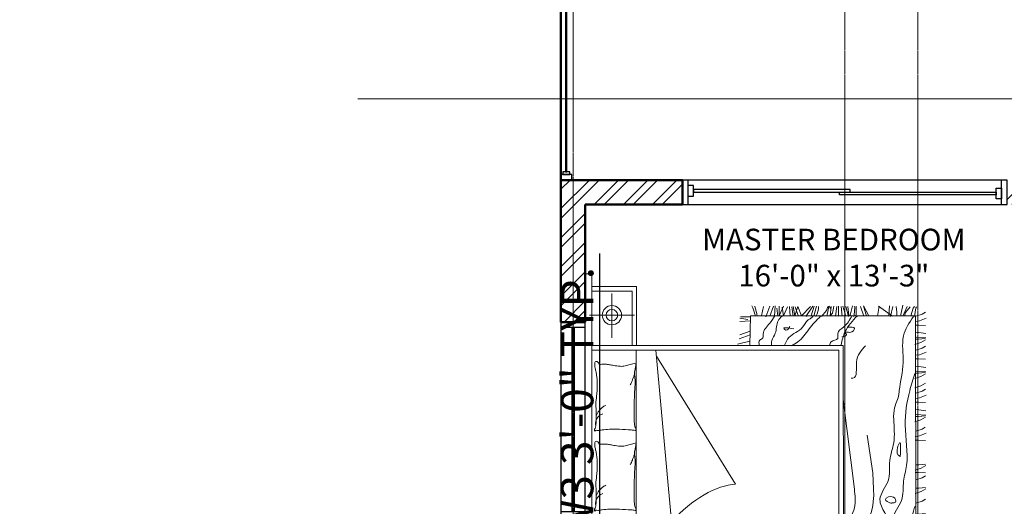
# Model space of a CAD drawing. Units: inches. Extents: x 261 to 2725, y 291 to 1454.
# Tile 22 of 35: x 1043 to 1407, y 853 to 1033. Entities that reach past the tile are written whole.
import ezdxf

# ---------------------------------------------------------------- set-up
doc = ezdxf.new("R2010")
doc.units = ezdxf.units.IN
doc.linetypes.add('CENTER', pattern=[2, 1.25, -0.25, 0.25, -0.25])
for name, color, linetype, lineweight in [('A-ANNO-DIMS', 136, 'Continuous', 18), ('A-AREA-IDEN', 18, 'Continuous', 18), ('A-DOOR', 160, 'Continuous', 25), ('A-FLOR-HRAL', 132, 'Continuous', 25), ('A-FURN', 30, 'Continuous', 18), ('A-GLAZ', 150, 'Continuous', 25), ('A-GRID', 251, 'CENTER', 13), ('A-WALL', 222, 'Continuous', 50), ('A-WALL-PATT', 243, 'Continuous', 13)]:
    doc.layers.add(name, color=color, linetype=linetype, lineweight=lineweight)
doc.styles.get("Standard").update_dxf_attribs({"font": 'arial.ttf'})
doc.dimstyles.new('ISO-25', dxfattribs={"dimtxt": 12, "dimasz": 6, "dimexe": 1.25, "dimexo": 0.625, "dimtad": 1, "dimdec": 0, "dimlunit": 3, "dimtxsty": 'Standard', "dimblk": 'ARCHTICK', "dimcen": 2.5, "dimadec": 0, "dimazin": 0, "dimtfac": 1, "dimtdec": 0, "dimtmove": 0, "dimatfit": 3, "dimfxl": 1, "dimfxlon": 1, "dimarcsym": 0})

# ---------------------------------------------------------------- blocks, each defined once
blk = doc.blocks.new('A$C2B723114')
for p, q in [((0, 2.9047), (2.8274, 2.9047)), ((0, 2.8487), (0, 2.9047)), ((0.4243, 2.8697), (0.4243, 2.4855)), ((2.4742, 2.8697), (2.4742, 2.4855)), ((2.8274, 2.9047), (2.8274, 2.8487)), ((2.8274, 2.8487), (0, 2.8487)), ((0.1012, 2.4649), (0.1012, 2.849)), ((0.1396, 2.5033), (0.1396, 2.849)), ((0.6794, 0.7051), (0.6794, 2.8509)), ((0.7187, 0.7435), (0.7187, 2.8509)), ((2.1776, 2.8509), (2.1776, 0.7454)), ((2.216, 2.8509), (2.216, 0.707)), ((2.6798, 2.5052), (2.6798, 2.8509)), ((2.7182, 2.4668), (2.7182, 2.8509)), ((0.6087, 2.6776), (0.295, 2.6776)), ((2.6586, 2.6776), (2.2821, 2.6776)), ((1.3789, 2.4999), (1.3598, 2.5761)), ((2.0593, 2.4999), (2.0402, 2.5761)), ((0.6794, 2.4649), (0.1012, 2.4649)), ((0.6766, 2.5033), (0.1396, 2.5033)), ((0.7191, 2.47), (2.1778, 2.4719)), ((1.3858, 2.4723), (1.3789, 2.4999)), ((2.0662, 2.4723), (2.0593, 2.4999)), ((2.2188, 2.5052), (2.6798, 2.5052)), ((2.2188, 2.4668), (2.7182, 2.4668)), ((2.1771, 2.3036), (0.718, 2.1685)), ((1.0365, 1.6233), (2.1246, 2.2989)), ((2.2287, 1.6076), (2.2523, 1.5035)), ((0.5047, 1.5819), (0.5353, 1.4945)), ((0.6174, 1.5819), (0.6232, 1.4916)), ((0.6467, 1.5819), (0.6369, 1.5137)), ((0.6571, 1.4945), (0.6571, 1.5765)), ((2.2726, 1.593), (2.3061, 1.5007)), ((2.3067, 1.5881), (2.3373, 1.5007)), ((2.4194, 1.5881), (2.4251, 1.4979)), ((2.4487, 1.5881), (2.4389, 1.5199)), ((2.4591, 1.5007), (2.4591, 1.5828)), ((0.4269, 0.0884), (0.4269, 1.4945)), ((0.4269, 1.4945), (0.6794, 1.4945)), ((2.4685, 1.4964), (2.216, 1.5022)), ((2.4685, 1.4964), (2.4685, 0.0903)), ((0.3172, 1.3923), (0.4213, 1.3687)), ((0.3318, 1.3485), (0.4241, 1.3149)), ((2.4596, 1.3659), (2.552, 1.3324)), ((2.4685, 1.4044), (2.5491, 1.3861)), ((0.3367, 1.3143), (0.4241, 1.2838)), ((2.4645, 1.3318), (2.552, 1.3012)), ((2.4645, 1.2928), (2.5548, 1.2871)), ((2.4645, 1.2635), (2.5328, 1.2733)), ((0.3367, 1.2016), (0.427, 1.1959)), ((0.3367, 1.1724), (0.405, 1.1821)), ((2.4699, 1.2531), (2.552, 1.2163)), ((2.552, 1.2531), (2.4699, 1.2531)), ((2.5435, 1.2276), (2.4699, 1.2163)), ((2.4699, 1.2163), (2.5463, 1.1823)), ((0.4241, 1.162), (0.3421, 1.162)), ((0.3421, 1.162), (0.4241, 1.1252)), ((2.5491, 1.1654), (2.467, 1.1597)), ((2.5463, 1.1455), (2.467, 1.1342)), ((2.5491, 1.1342), (2.4699, 1.1201)), ((2.4699, 1.1201), (2.5491, 1.0946)), ((2.5491, 1.0946), (2.4699, 1.0635)), ((2.5463, 1.1172), (2.4727, 1.0918)), ((0.4157, 1.0206), (0.3421, 1.0093)), ((0.3421, 1.0093), (0.4185, 0.9754)), ((2.4642, 1.0267), (2.552, 0.9644)), ((2.4699, 1.0635), (2.5491, 0.9842)), ((0.4213, 0.9584), (0.3392, 0.9527)), ((0.4185, 0.9386), (0.3392, 0.9272)), ((0.4213, 0.9272), (0.3421, 0.9131)), ((2.4642, 0.9389), (2.4869, 0.9276)), ((2.467, 0.9559), (2.552, 0.9333)), ((2.4699, 0.9785), (2.552, 0.9531)), ((2.4869, 0.9276), (2.5265, 0.9163)), ((0.3421, 0.9131), (0.4213, 0.8876)), ((0.4213, 0.8876), (0.3421, 0.8565)), ((0.3421, 0.8565), (0.4213, 0.7772)), ((0.4185, 0.9103), (0.3449, 0.8848)), ((2.4642, 0.8908), (2.5152, 0.8483)), ((2.467, 0.8455), (2.5208, 0.8342)), ((2.5152, 0.8483), (2.5491, 0.837)), ((2.5265, 0.9163), (2.5491, 0.9163)), ((0.3364, 0.8197), (0.4241, 0.7574)), ((0.3421, 0.7716), (0.4241, 0.7461)), ((2.5491, 0.7606), (2.467, 0.7719)), ((2.4699, 0.8172), (2.4925, 0.7974)), ((2.5491, 0.8087), (2.4699, 0.8172)), ((2.4925, 0.7974), (2.535, 0.7889)), ((2.5208, 0.8342), (2.552, 0.8285)), ((2.552, 0.8285), (2.5293, 0.8087)), ((2.535, 0.7889), (2.552, 0.7861)), ((0.3392, 0.7489), (0.4241, 0.7263)), ((0.359, 0.7206), (0.3987, 0.7093)), ((0.3987, 0.7093), (0.4213, 0.7093)), ((2.216, 0.707), (0.6794, 0.7051)), ((2.1776, 0.7454), (0.7187, 0.7435)), ((0.9938, 0.6115), (1.7555, 0.7064)), ((2.5491, 0.6842), (2.4642, 0.6615)), ((2.4727, 0.7464), (2.467, 0.7408)), ((2.467, 0.7153), (2.5491, 0.7238)), ((2.552, 0.7096), (2.467, 0.6842)), ((2.552, 0.7464), (2.4727, 0.7464)), ((0.3364, 0.6233), (0.4241, 0.561)), ((0.3421, 0.6601), (0.4213, 0.5808)), ((2.4642, 0.6191), (2.4784, 0.6134)), ((2.467, 0.5993), (2.4869, 0.5964)), ((2.5491, 0.6672), (2.4755, 0.6587)), ((2.4755, 0.6474), (2.5548, 0.6276)), ((2.4784, 0.6134), (2.5406, 0.6077)), ((2.4869, 0.5964), (2.552, 0.5964)), ((2.5406, 0.6077), (2.552, 0.6134)), ((0.3392, 0.5525), (0.4241, 0.5299)), ((0.3421, 0.5752), (0.4241, 0.5497)), ((0.359, 0.5242), (0.3987, 0.5129)), ((2.467, 0.5313), (2.5491, 0.5596)), ((2.467, 0.5087), (2.5548, 0.5342)), ((2.5548, 0.5342), (2.4699, 0.4889)), ((0.3364, 0.4785), (0.3874, 0.436)), ((0.3392, 0.4332), (0.393, 0.4219)), ((0.3874, 0.436), (0.4213, 0.4247)), ((0.393, 0.4219), (0.4241, 0.4162)), ((1.1305, 0.4537), (0.9938, 0.448)), ((1.4523, 0.5021), (1.1305, 0.4537)), ((0.4213, 0.415), (0.3364, 0.3923)), ((0.4241, 0.2868), (0.3392, 0.415)), ((0.4213, 0.3377), (0.3392, 0.3491)), ((0.3421, 0.4049), (0.3647, 0.3851)), ((0.4213, 0.3964), (0.3421, 0.4049)), ((0.4213, 0.398), (0.3477, 0.3895)), ((0.3647, 0.3851), (0.4072, 0.3766)), ((0.4241, 0.4162), (0.4015, 0.3964)), ((0.4072, 0.3766), (0.4241, 0.3738)), ((2.467, 0.4133), (2.552, 0.4019)), ((2.467, 0.2879), (2.552, 0.4076)), ((0.3392, 0.2925), (0.4213, 0.3009)), ((0.4241, 0.3236), (0.3449, 0.3236)), ((0.3477, 0.2571), (0.427, 0.2373)), ((2.4642, 0.3049), (2.5491, 0.2851)), ((2.467, 0.319), (2.5548, 0.3134)), ((2.501, 0.2491), (2.5491, 0.2547)), ((0.3506, 0.2231), (0.4128, 0.2175)), ((0.359, 0.2061), (0.4241, 0.2061)), ((0.4128, 0.2175), (0.4241, 0.2231)), ((2.467, 0.2179), (2.5605, 0.1981)), ((2.467, 0.1981), (2.5491, 0.1613)), ((2.467, 0.184), (2.4982, 0.1755)), ((2.4699, 0.2491), (2.501, 0.2491)), ((2.4982, 0.1755), (2.5463, 0.1359)), ((0.3392, 0.1042), (0.4213, 0.1325)), ((0.3392, 0.0815), (0.427, 0.107)), ((0.427, 0.107), (0.3421, 0.0617)), ((2.4685, 0.0903), (0.4269, 0.0884)), ((0.5106, 0.094), (0.5106, 0.0657)), ((0.5417, 0.094), (0.5474, 0.0572)), ((0.587, 0.0884), (0.604, 0.0346)), ((0.6512, 0.0884), (0.6682, 0.0346)), ((0.713, 0.094), (0.713, 0.0657)), ((0.7334, 0.0943), (0.7503, 0.0434)), ((0.7786, 0.0915), (0.7786, 0.0632)), ((0.8739, 0.0884), (0.8908, 0.0346)), ((0.956, 0.0943), (0.973, 0.0434)), ((1.0013, 0.0915), (1.0013, 0.0632)), ((1.072, 0.0884), (1.089, 0.0346)), ((1.1338, 0.094), (1.1338, 0.0657)), ((1.1542, 0.0943), (1.1712, 0.0434)), ((1.1995, 0.0915), (1.1995, 0.0632)), ((1.4088, 0.094), (1.4088, 0.0657)), ((1.44, 0.094), (1.4456, 0.0572)), ((1.4853, 0.0884), (1.5023, 0.0346)), ((1.5674, 0.0962), (1.5844, 0.0453)), ((1.6127, 0.0934), (1.6127, 0.0651)), ((1.6297, 0.0849), (1.624, 0.0028)), ((1.6721, 0.0877), (1.6693, 0.0623)), ((1.7344, 0.0934), (1.7344, 0.0651)), ((1.7655, 0.0934), (1.7712, 0.0566)), ((1.8108, 0.0877), (1.8278, 0.034)), ((1.8568, 0.0962), (1.8738, 0.0453)), ((1.9342, 0.0962), (1.9512, 0.0453)), ((1.9795, 0.0934), (1.9795, 0.0651)), ((1.9965, 0.0849), (1.9908, 0.0028)), ((2.039, 0.0877), (2.0361, 0.0623)), ((2.1012, 0.0934), (2.1012, 0.0651)), ((2.1324, 0.0934), (2.138, 0.0566)), ((2.1777, 0.0877), (2.1946, 0.034)), ((2.2236, 0.0962), (2.2406, 0.0453)), ((2.2689, 0.0934), (2.2689, 0.0651)), ((2.2859, 0.0849), (2.2802, 0.0028)), ((2.3284, 0.0877), (2.3255, 0.0623)), ((2.3906, 0.0934), (2.3906, 0.0651)), ((2.4218, 0.0934), (2.4274, 0.0566)), ((2.4642, 0.0991), (2.5378, 0.0877)), ((2.467, 0.0877), (2.484, 0.034)), ((2.4699, 0.1302), (2.535, 0.1104)), ((2.535, 0.1104), (2.5491, 0.0991)), ((2.5378, 0.0877), (2.5463, 0.0821)), ((0.5106, 0.0657), (0.5077, 0.0063)), ((0.5474, 0.0572), (0.57, 0.0006)), ((0.604, 0.0346), (0.621, 0.0063)), ((0.6682, 0.0346), (0.6851, 0.0063)), ((0.713, 0.0657), (0.7101, 0.0063)), ((0.7503, 0.0434), (0.773, 0.0037)), ((0.7786, 0.0632), (0.7843, 0.0066)), ((0.8908, 0.0346), (0.9078, 0.0063)), ((0.973, 0.0434), (0.9957, 0.0037)), ((1.0013, 0.0632), (1.007, 0.0066)), ((1.089, 0.0346), (1.106, 0.0063)), ((1.1338, 0.0657), (1.131, 0.0063)), ((1.1712, 0.0434), (1.1939, 0.0037)), ((1.1995, 0.0632), (1.2052, 0.0066)), ((1.4088, 0.0657), (1.406, 0.0063)), ((1.4456, 0.0572), (1.4683, 0.0006)), ((1.5023, 0.0346), (1.5192, 0.0082)), ((1.5844, 0.0453), (1.607, 0.0057)), ((1.6127, 0.0651), (1.6184, 0.0085)), ((1.6693, 0.0623), (1.6608, 0.0028)), ((1.7344, 0.0651), (1.7316, 0.0057)), ((1.7712, 0.0566), (1.7938, 0)), ((1.8278, 0.034), (1.8448, 0.0057)), ((1.8738, 0.0453), (1.8964, 0.0057)), ((1.9512, 0.0453), (1.9739, 0.0057)), ((1.9795, 0.0651), (1.9852, 0.0085)), ((2.0361, 0.0623), (2.0276, 0.0028)), ((2.1012, 0.0651), (2.0984, 0.0057)), ((2.138, 0.0566), (2.1607, 0)), ((2.1946, 0.034), (2.2116, 0.0057)), ((2.2406, 0.0453), (2.2632, 0.0057)), ((2.2689, 0.0651), (2.2746, 0.0085)), ((2.3255, 0.0623), (2.317, 0.0028)), ((2.3906, 0.0651), (2.3878, 0.0057)), ((2.4274, 0.0566), (2.4501, 0)), ((2.484, 0.034), (2.501, 0.0057))]:
    blk.add_line(p, q)
for centre, radius in [((0.4243, 2.6776), 0.0821), ((0.4243, 2.6776), 0.0493), ((2.4742, 2.6776), 0.0821), ((2.4742, 2.6776), 0.0493)]:
    blk.add_circle(centre, radius)
for centre, radius, start, end in [((0.8078, 2.821), 0.00214, 160.43603, 281.89306), ((0.8088, 2.8207), 0.00315, 111.7883, 160.43603), ((0.8162, 2.8021), 0.0232, 94.30254, 111.7883), ((0.8091, 2.8151), 0.00394, 21.9904, 101.89306), ((0.8409, 2.7949), 0.0302, 158.57902, 188.13348), ((1.0356, 2.8227), 0.2268, 188.13348, 192.10946), ((0.7994, 2.8112), 0.0144, 338.57902, 21.9904), ((0.635, 2.7368), 0.1829, 7.6809, 12.10946), ((0.8165, 2.7987), 0.0266, 59.34875, 94.30254), ((0.8554, 2.8643), 0.0497, 239.34875, 264.74081), ((0.9202, 3.5684), 0.7568, 264.74081, 268.09211), ((0.8679, 2.7254), 0.0915, 74.06476, 94.21588), ((0.8679, 2.7254), 0.0915, 53.91364, 74.06476), ((0.9409, 4.189), 1.3777, 268.09211, 270.57574), ((0.8679, 2.7254), 0.0915, 36.17665, 53.91364), ((0.86, 2.6097), 0.2158, 62.76041, 69.13972), ((0.8679, 2.7254), 0.0915, 18.43965, 36.17665), ((0.9466, 3.6164), 0.8051, 270.57574, 274.80185), ((0.9263, 2.7386), 0.0708, 51.61143, 62.76041), ((0.7461, 2.511), 0.3611, 46.18849, 51.61143), ((0.8523, 2.6218), 0.2076, 39.03494, 46.18849), ((1.0364, 2.548), 0.2671, 87.46141, 94.80185), ((1.042, 2.6745), 0.1405, 79.81012, 87.46141), ((1.1532, 3.2931), 0.488, 259.81012, 263.9133), ((1.204, 3.7695), 0.9671, 263.9133, 270), ((1.204, 3.4318), 0.6294, 270, 277.54685), ((1.2573, 3.0292), 0.2233, 277.54685, 285.74398), ((1.3941, 2.5438), 0.281, 98.43719, 105.74398), ((1.3747, 2.6748), 0.1486, 90, 98.43719), ((1.3713, 2.8186), 0.0315, 274.40021, 333.41948), ((0.923, 2.7382), 0.4535, 0, 6.23236), ((1.3747, 2.74), 0.0833, 78.72762, 90), ((1.3886, 2.8099), 0.0121, 333.41948, 78.72762), ((1.4882, 2.821), 0.00214, 160.43603, 281.89306), ((1.4892, 2.8207), 0.00315, 111.7883, 160.43603), ((1.4966, 2.8021), 0.0232, 94.30254, 111.7883), ((1.4895, 2.8151), 0.00394, 21.9904, 101.89306), ((1.5213, 2.7949), 0.0302, 158.57902, 188.13348), ((1.716, 2.8227), 0.2268, 188.13348, 192.10946), ((1.4798, 2.8112), 0.0144, 338.57902, 21.9904), ((1.3154, 2.7368), 0.1829, 7.6809, 12.10946), ((1.4969, 2.7987), 0.0266, 59.34875, 94.30254), ((1.5358, 2.8643), 0.0497, 239.34875, 264.74081), ((1.6006, 3.5684), 0.7568, 264.74081, 268.09211), ((1.5483, 2.7254), 0.0915, 74.06476, 94.21588), ((1.5483, 2.7254), 0.0915, 53.91364, 74.06476), ((1.6213, 4.189), 1.3777, 268.09211, 270.57574), ((1.5483, 2.7254), 0.0915, 36.17665, 53.91364), ((1.5404, 2.6097), 0.2158, 62.76041, 69.13972), ((1.5483, 2.7254), 0.0915, 18.43965, 36.17665), ((1.627, 3.6164), 0.8051, 270.57574, 274.80185), ((1.6067, 2.7386), 0.0708, 51.61143, 62.76041), ((1.4265, 2.511), 0.3611, 46.18849, 51.61143), ((1.5327, 2.6218), 0.2076, 39.03494, 46.18849), ((1.7168, 2.548), 0.2671, 87.46141, 94.80185), ((1.7224, 2.6745), 0.1405, 79.81012, 87.46141), ((1.8336, 3.2931), 0.488, 259.81012, 263.9133), ((1.8844, 3.7695), 0.9671, 263.9133, 270), ((1.8844, 3.4318), 0.6294, 270, 277.54685), ((1.9377, 3.0292), 0.2233, 277.54685, 285.74398), ((2.0745, 2.5438), 0.281, 98.43719, 105.74398), ((2.0551, 2.6748), 0.1486, 90, 98.43719), ((2.0517, 2.8186), 0.0315, 274.40021, 333.41948), ((1.6034, 2.7382), 0.4535, 0, 6.23236), ((2.0551, 2.74), 0.0833, 78.72762, 90), ((2.069, 2.8099), 0.0121, 333.41948, 78.72762), ((-0.0181, 2.6487), 0.8418, 3.36875, 7.6809), ((0.1976, 2.6614), 0.6258, 358.36691, 3.36875), ((0.9783, 2.7239), 0.0455, 28.31676, 39.03494), ((0.8558, 2.6579), 0.1846, 23.00277, 28.31676), ((0.5722, 2.8434), 0.8132, 347.80162, 350.31563), ((1.1884, 2.7382), 0.1881, 350.31563, 0), ((0.6623, 2.6487), 0.8418, 3.36875, 7.6809), ((0.878, 2.6614), 0.6258, 358.36691, 3.36875), ((1.6587, 2.7239), 0.0455, 28.31676, 39.03494), ((1.5362, 2.6579), 0.1846, 23.00277, 28.31676), ((1.2526, 2.8434), 0.8132, 347.80162, 350.31563), ((1.8688, 2.7382), 0.1881, 350.31563, 0), ((-11.7321, 3.2823), 12.5718, 356.49514, 356.94504), ((-0.4351, 2.6794), 1.2587, 356.94504, 358.36691), ((1.9648, 2.5659), 0.6074, 171.99495, 177.33512), ((1.6528, 2.6098), 0.2924, 167.80162, 171.99495), ((-11.0517, 3.2823), 12.5718, 356.49514, 356.94504), ((0.2453, 2.6794), 1.2587, 356.94504, 358.36691), ((2.6452, 2.5659), 0.6074, 171.99495, 177.33512), ((2.3332, 2.6098), 0.2924, 167.80162, 171.99495), ((1.4917, 3.1364), 0.681, 244.68893, 246.51559), ((1.4204, 2.5912), 0.0624, 177.33512, 194.04519), ((2.1721, 3.1364), 0.681, 244.68893, 246.51559), ((2.1008, 2.5912), 0.0624, 177.33512, 194.04519), ((0.8298, 2.4774), 0.0178, 170.00164, 196.69777), ((0.5206, 2.5319), 0.2961, 350.00164, 356.49514), ((0.8139, 2.4726), 0.00122, 196.69777, 277.12039), ((0.8041, 2.5514), 0.0807, 277.12039, 286.22115), ((0.8068, 2.5419), 0.0707, 286.22115, 297.28412), ((0.8584, 2.4419), 0.0418, 102.86904, 117.28412), ((0.879, 2.3515), 0.1345, 93.57397, 102.86904), ((0.9376, 1.4146), 1.0732, 90.28654, 93.57397), ((0.9586, -2.7845), 5.2724, 89.02962, 90.28654), ((0.9954, -0.6123), 3.0999, 87.39037, 89.02962), ((1.0854, 1.364), 1.1216, 85.38242, 87.39037), ((1.28, 3.7729), 1.2952, 265.38242, 267.25094), ((1.228, 2.691), 0.2121, 267.25094, 281.55856), ((1.4917, 3.1364), 0.681, 246.51559, 248.34226), ((1.4917, 3.1364), 0.681, 248.34226, 250.57202), ((1.4917, 3.1364), 0.681, 250.57202, 252.80178), ((1.2975, 2.3514), 0.1345, 83.56595, 101.55856), ((1.3002, 2.3754), 0.1104, 72.61359, 83.56595), ((1.3965, 2.6828), 0.2118, 252.61359, 260.5159), ((1.4027, 2.7202), 0.2496, 260.5159, 265.91706), ((1.385, 2.4721), 0.000845, 265.91706, 14.04494), ((1.5102, 2.4774), 0.0178, 170.00164, 196.69777), ((1.201, 2.5319), 0.2961, 350.00164, 356.49514), ((1.4943, 2.4726), 0.00122, 196.69777, 277.12039), ((1.4845, 2.5514), 0.0807, 277.12039, 286.22115), ((1.4872, 2.5419), 0.0707, 286.22115, 297.28412), ((1.5388, 2.4419), 0.0418, 102.86904, 117.28412), ((1.5594, 2.3515), 0.1345, 93.57397, 102.86904), ((1.618, 1.4146), 1.0732, 90.28654, 93.57397), ((1.639, -2.7845), 5.2724, 89.02962, 90.28654), ((1.6758, -0.6123), 3.0999, 87.39037, 89.02962), ((1.7658, 1.364), 1.1216, 85.38242, 87.39037), ((1.9604, 3.7729), 1.2952, 265.38242, 267.25094), ((1.9084, 2.691), 0.2121, 267.25094, 281.55856), ((2.1721, 3.1364), 0.681, 246.51559, 248.34226), ((2.1721, 3.1364), 0.681, 248.34226, 250.57202), ((2.1721, 3.1364), 0.681, 250.57202, 252.80178), ((1.9779, 2.3514), 0.1345, 83.56595, 101.55856), ((1.9806, 2.3754), 0.1104, 72.61359, 83.56595), ((2.0769, 2.6828), 0.2118, 252.61359, 260.5159), ((2.0831, 2.7202), 0.2496, 260.5159, 265.91706), ((2.0654, 2.4721), 0.000845, 265.91706, 14.04494)]:
    blk.add_arc(centre, radius, start, end)
blk.add_ellipse((0.4962, 1.9132), major_axis=(0.4887, -0.4605), ratio=0.503305, start_param=0.491272, end_param=1.591113)
for points, knots in [([(0.427, 1.4678), (0.4036, 1.4582), (0.3693, 1.4441), (0.3335, 1.4344), (0.3221, 1.4313)], [0, 0, 0, 0, 98.452083, 144.639601, 144.639601, 144.639601, 144.639601]), ([(0.4241, 1.4423), (0.4031, 1.437), (0.3691, 1.4284), (0.3351, 1.4199), (0.3221, 1.4167)], [0, 0, 0, 0, 84.638756, 136.955563, 136.955563, 136.955563, 136.955563]), ([(0.6768, 1.3104), (0.6615, 1.3339), (0.6315, 1.3797), (0.604, 1.4501), (0.5417, 1.4748), (0.5064, 1.4871), (0.4848, 1.4945)], [0, 0, 0, 0, 110.980521, 216.571322, 273.316778, 363.252298, 363.252298, 363.252298, 363.252298]), ([(2.2145, 1.4211), (2.233, 1.4246), (2.2636, 1.4303), (2.2761, 1.3837), (2.3429, 1.3967), (2.3949, 1.3342), (2.4474, 1.3031), (2.4698, 1.2898)], [0, 0, 0, 0, 61.886907, 102.717887, 145.699352, 284.082577, 386.765171, 386.765171, 386.765171, 386.765171]), ([(2.5548, 1.4853), (2.5314, 1.4757), (2.5031, 1.4641), (2.4737, 1.4555), (2.4685, 1.454)], [0, 0, 0, 0, 98.452083, 119.481049, 119.481049, 119.481049, 119.481049]), ([(2.552, 1.4598), (2.5309, 1.4545), (2.5031, 1.4475), (2.4753, 1.4406), (2.4685, 1.4389)], [0, 0, 0, 0, 84.638756, 111.94623, 111.94623, 111.94623, 111.94623]), ([(0.6768, 1.286), (0.6567, 1.2911), (0.6145, 1.3017), (0.5543, 1.3533), (0.4816, 1.349), (0.4362, 1.3493), (0.4233, 1.3493)], [0, 0, 0, 0, 80.250278, 168.388677, 295.908361, 346.663112, 346.663112, 346.663112, 346.663112]), ([(0.4233, 1.3445), (0.4367, 1.3385), (0.464, 1.3264), (0.5129, 1.2848), (0.5456, 1.2161), (0.6131, 1.2349), (0.6142, 1.1913), (0.6642, 1.1806), (0.674, 1.144), (0.6817, 1.1154)], [0, 0, 0, 0, 56.745495, 115.23739, 254.956954, 286.678662, 337.828324, 366.201072, 468.500395, 468.500395, 468.500395, 468.500395]), ([(2.2145, 1.319), (2.2295, 1.319), (2.2678, 1.3192), (2.3288, 1.2705), (2.4143, 1.279), (2.4535, 1.2403), (2.4662, 1.2278)], [0, 0, 0, 0, 57.155505, 146.33427, 287.936209, 355.396728, 355.396728, 355.396728, 355.396728]), ([(2.2182, 1.2059), (2.2419, 1.1958), (2.3116, 1.1659), (2.342, 1.0552), (2.4266, 1.0223), (2.4474, 0.9811), (2.462, 0.9684), (2.4698, 0.9616)], [0, 0, 0, 0, 97.73655, 287.59661, 389.176293, 423.403759, 463.679181, 463.679181, 463.679181, 463.679181]), ([(2.3573, 1.127), (2.3656, 1.1759), (2.3758, 1.2352), (2.3371, 1.1853), (2.3602, 1.1713), (2.3768, 1.1612)], [0, 0, 0, 0, 107.853607, 130.728419, 189.220329, 189.220329, 189.220329, 189.220329]), ([(2.2145, 1.1476), (2.2246, 1.1286), (2.2575, 1.0666), (2.3612, 1.0009), (2.431, 0.9336), (2.4662, 0.8996)], [0, 0, 0, 0, 83.02987, 271.460712, 463.033803, 463.033803, 463.033803, 463.033803]), ([(0.6817, 0.8034), (0.6673, 0.8119), (0.6341, 0.8315), (0.5785, 0.8518), (0.5349, 0.8973), (0.4828, 0.9461), (0.4518, 0.9879), (0.4331, 1.013)], [0, 0, 0, 0, 65.318952, 150.437229, 226.833166, 307.58338, 429.454095, 429.454095, 429.454095, 429.454095]), ([(0.4282, 0.9448), (0.4547, 0.9353), (0.496, 0.9206), (0.5223, 0.8436), (0.5628, 0.7946), (0.6113, 0.7575), (0.6214, 0.7173), (0.6539, 0.7022), (0.672, 0.6897), (0.6768, 0.6864)], [0, 0, 0, 0, 102.299436, 159.044876, 303.717955, 348.579152, 391.138254, 454.581655, 477.456496, 477.456496, 477.456496, 477.456496]), ([(2.2145, 0.823), (2.227, 0.8201), (2.261, 0.8121), (2.261, 0.7401), (2.3352, 0.7659), (2.379, 0.6836), (2.4336, 0.6521), (2.4662, 0.6334)], [0, 0, 0, 0, 46.747668, 127.438174, 179.649794, 280.561838, 429.605131, 429.605131, 429.605131, 429.605131]), ([(0.4282, 0.74), (0.4347, 0.7029), (0.444, 0.6496), (0.5194, 0.6274), (0.555, 0.5807), (0.5975, 0.5243), (0.6789, 0.5415), (0.677, 0.5095), (0.6768, 0.5061)], [0, 0, 0, 0, 130.791737, 187.537266, 286.231946, 353.673191, 460.023761, 472.712403, 472.712403, 472.712403, 472.712403]), ([(0.6768, 0.6864), (0.7275, 0.655), (0.8251, 0.5944), (0.9391, 0.606), (0.9938, 0.6115)], [0, 0, 0, 0, 225.995823, 434.686543, 434.686543, 434.686543, 434.686543]), ([(2.2218, 0.7246), (2.2595, 0.716), (2.3548, 0.6945), (2.4265, 0.6268), (2.4698, 0.586)], [0, 0, 0, 0, 148.665024, 375.555892, 375.555892, 375.555892, 375.555892]), ([(2.3719, 0.6737), (2.3738, 0.6431), (2.3772, 0.5878), (2.3146, 0.6382), (2.3401, 0.7015), (2.2971, 0.6649), (2.2923, 0.6965), (2.289, 0.7176)], [0, 0, 0, 0, 83.446591, 150.887818, 201.642461, 230.015204, 286.760644, 286.760644, 286.760644, 286.760644]), ([(2.2145, 0.5167), (2.1764, 0.5522), (2.1051, 0.6184), (1.9357, 0.5803), (1.9385, 0.6342), (1.9388, 0.6395)], [0, 0, 0, 0, 208.073343, 389.01094, 409.01094, 409.01094, 409.01094, 409.01094]), ([(0.6768, 0.5061), (0.7554, 0.4794), (0.8591, 0.4442), (0.9675, 0.4473), (0.9938, 0.448)], [0, 0, 0, 0, 319.374611, 421.61723, 421.61723, 421.61723, 421.61723]), ([(0.4331, 0.4427), (0.4498, 0.4356), (0.4827, 0.4216), (0.5314, 0.3759), (0.632, 0.3884), (0.6996, 0.3513), (0.7423, 0.3278)], [0, 0, 0, 0, 70.931849, 139.556414, 248.154027, 434.709995, 434.709995, 434.709995, 434.709995]), ([(2.4625, 0.1088), (2.4095, 0.1438), (2.2904, 0.2226), (2.0623, 0.1771), (1.9006, 0.2246), (1.7699, 0.2337), (1.6941, 0.2766), (1.5528, 0.2786), (1.4005, 0.2587), (1.2324, 0.3267), (1.059, 0.2939), (0.9218, 0.426), (0.7359, 0.3204), (0.5586, 0.2391), (0.4502, 0.3116), (0.427, 0.3272)], [0, 0, 0, 0, 239.874704, 538.942419, 850.40885, 893.390315, 1047.998294, 1176.505142, 1437.500972, 1637.333004, 1864.324391, 2089.058767, 2248.736533, 2637.953392, 2744.252142, 2744.252142, 2744.252142, 2744.252142]), ([(1.9771, 0.0962), (1.9286, 0.1117), (1.7864, 0.157), (1.5223, 0.1992), (1.2611, 0.141), (1.0527, 0.2023), (0.8859, 0.1885), (0.76, 0.3042), (0.6211, 0.292), (0.5187, 0.3203), (0.4572, 0.3456), (0.4282, 0.3575)], [0, 0, 0, 0, 198.710624, 582.73994, 1031.873213, 1206.082894, 1423.278209, 1655.952104, 1808.744089, 1945.69963, 2068.229211, 2068.229211, 2068.229211, 2068.229211]), ([(0.8718, 0.2941), (0.8821, 0.3221), (0.9041, 0.3814), (0.9523, 0.2773), (0.8733, 0.2454), (0.8757, 0.2798), (0.8766, 0.2941)], [0, 0, 0, 0, 82.720021, 175.094899, 237.579423, 282.440623, 282.440623, 282.440623, 282.440623]), ([(0.8474, 0.0943), (0.82, 0.1047), (0.757, 0.1287), (0.6201, 0.1029), (0.4623, 0.1837), (0.4372, 0.2936), (0.4282, 0.3331)], [0, 0, 0, 0, 112.422038, 258.341957, 533.791494, 688.286079, 688.286079, 688.286079, 688.286079]), ([(1.2715, 0.221), (1.3344, 0.2172), (1.4529, 0.21), (1.2971, 0.2665), (1.2756, 0.2284), (1.2715, 0.221)], [0, 0, 0, 0, 150.888188, 283.977876, 315.699589, 315.699589, 315.699589, 315.699589])]:
    blk.add_open_spline(points, degree=3, knots=knots)
blk = doc.blocks.new('WIN-72')
for p, q in [((955.45, 950.47), (946.45, 950.47)), ((950.45, 950.47), (950.45, 882.47)), ((951.45, 882.47), (951.45, 950.47)), ((946.45, 882.47), (955.45, 882.47))]:
    blk.add_line(p, q)
blk.add_lwpolyline([(955.45, 880.47), (955.45, 952.47), (946.45, 952.47), (946.45, 880.47)], close=True)
blk = doc.blocks.new('_ArchTick')
at = {"color": 0, "linetype": 'ByBlock', "const_width": 0.15}
blk.add_lwpolyline([(-0.5, -0.5), (0.5, 0.5)], dxfattribs=at)
blk = doc.blocks.new('*D59')
at = {"layer": 'A-ANNO-DIMS', "color": 0, "lineweight": -2, "ltscale": 0.07, "transparency": 16777216}
for p, q in [((1257.48, 757.47), (1257.48, 946.37)), ((1256.48, 757.47), (1258.73, 757.47)), ((1257.48, 721.47), (1257.48, 757.47)), ((1256.48, 721.47), (1258.73, 721.47))]:
    blk.add_line(p, q, dxfattribs=at)
at = {"layer": 'Defpoints', "color": 0, "ltscale": 0.07, "transparency": 16777216}
for p in [(1252.08, 757.47), (1257.48, 757.47), (1252.08, 721.47)]:
    blk.add_point(p, dxfattribs=at)
at = {"layer": 'A-ANNO-DIMS', "color": 0, "lineweight": -2, "ltscale": 0.07, "transparency": 16777216, "xscale": 6, "yscale": 6, "zscale": 6}
for p, rotation in [((1257.48, 757.47), 90), ((1257.48, 721.47), 270)]:
    blk.add_blockref('_ArchTick', p, dxfattribs=dict(at, rotation=rotation))
at = {"layer": 'A-ANNO-DIMS', "color": 0, "ltscale": 0.07, "transparency": 16777216, "insert": (1250.64, 854.92), "char_height": 12, "attachment_point": 5, "rotation": 90}
blk.add_mtext('WINDOW W3 3\'-0" TYP.', dxfattribs=at)
blk = doc.blocks.new('*D84')
at = {"layer": 'A-ANNO-DIMS', "color": 0, "lineweight": -2, "ltscale": 0.07, "transparency": 16777216}
for p, q in [((2600.96, 1024.47), (2603.21, 1024.47)), ((2601.96, 799.47), (2601.96, 1024.47)), ((2600.96, 799.47), (2603.21, 799.47))]:
    blk.add_line(p, q, dxfattribs=at)
at = {"layer": 'Defpoints', "color": 0, "ltscale": 0.07, "transparency": 16777216}
for p in [(946.45, 1024.47), (2601.96, 1024.47), (946.45, 799.47)]:
    blk.add_point(p, dxfattribs=at)
at = {"layer": 'A-ANNO-DIMS', "color": 0, "lineweight": -2, "ltscale": 0.07, "transparency": 16777216, "xscale": 6, "yscale": 6, "zscale": 6}
for p, rotation in [((2601.96, 1024.47), 90), ((2601.96, 799.47), 270)]:
    blk.add_blockref('_ArchTick', p, dxfattribs=dict(at, rotation=rotation))
at = {"layer": 'A-ANNO-DIMS', "color": 0, "ltscale": 0.07, "transparency": 16777216, "insert": (2595.21, 911.97), "char_height": 12, "attachment_point": 5, "rotation": 90}
blk.add_mtext('18\'-9"', dxfattribs=at)
blk = doc.blocks.new('*D85')
at = {"layer": 'A-ANNO-DIMS', "color": 0, "lineweight": -2, "ltscale": 0.07, "transparency": 16777216}
for p, q in [((2600.96, 1222.47), (2603.21, 1222.47)), ((2601.96, 1024.47), (2601.96, 1222.47)), ((2600.96, 1024.47), (2603.21, 1024.47))]:
    blk.add_line(p, q, dxfattribs=at)
at = {"layer": 'Defpoints', "color": 0, "ltscale": 0.07, "transparency": 16777216}
for p in [(946.45, 1222.47), (2601.96, 1222.47), (946.45, 1024.47)]:
    blk.add_point(p, dxfattribs=at)
at = {"layer": 'A-ANNO-DIMS', "color": 0, "lineweight": -2, "ltscale": 0.07, "transparency": 16777216, "xscale": 6, "yscale": 6, "zscale": 6}
for p, rotation in [((2601.96, 1222.47), 90), ((2601.96, 1024.47), 270)]:
    blk.add_blockref('_ArchTick', p, dxfattribs=dict(at, rotation=rotation))
at = {"layer": 'A-ANNO-DIMS', "color": 0, "ltscale": 0.07, "transparency": 16777216, "insert": (2595.21, 1123.47), "char_height": 12, "attachment_point": 5, "rotation": 90}
blk.add_mtext('16\'-6"', dxfattribs=at)
blk = doc.blocks.new('*D103')
at = {"layer": 'A-ANNO-DIMS', "color": 0, "lineweight": -2, "ltscale": 0.07, "transparency": 16777216}
for p, q in [((287.06, 1231.47), (284.81, 1231.47)), ((286.06, 439.47), (286.06, 1231.47)), ((287.06, 439.47), (284.81, 439.47))]:
    blk.add_line(p, q, dxfattribs=at)
at = {"layer": 'Defpoints', "color": 0, "ltscale": 0.07, "transparency": 16777216}
for p in [(286.06, 1231.47), (1243.08, 1231.47), (1243.08, 439.47)]:
    blk.add_point(p, dxfattribs=at)
at = {"layer": 'A-ANNO-DIMS', "color": 0, "lineweight": -2, "ltscale": 0.07, "transparency": 16777216, "xscale": 6, "yscale": 6, "zscale": 6}
for p, rotation in [((286.06, 1231.47), 90), ((286.06, 439.47), 270)]:
    blk.add_blockref('_ArchTick', p, dxfattribs=dict(at, rotation=rotation))
at = {"layer": 'A-ANNO-DIMS', "color": 0, "ltscale": 0.07, "transparency": 16777216, "insert": (279.3, 835.47), "char_height": 12, "attachment_point": 5, "rotation": 90}
blk.add_mtext('66\'-0"', dxfattribs=at)
blk = doc.blocks.new('*D109')
at = {"layer": 'A-ANNO-DIMS', "color": 0, "lineweight": -2, "ltscale": 0.07, "transparency": 16777216}
for p, q in [((287.06, 964.47), (284.81, 964.47)), ((286.06, 799.47), (286.06, 964.47)), ((287.06, 799.47), (284.81, 799.47))]:
    blk.add_line(p, q, dxfattribs=at)
at = {"layer": 'Defpoints', "color": 0, "ltscale": 0.07, "transparency": 16777216}
for p in [(286.06, 964.47), (1252.08, 964.47), (1252.08, 799.47)]:
    blk.add_point(p, dxfattribs=at)
at = {"layer": 'A-ANNO-DIMS', "color": 0, "lineweight": -2, "ltscale": 0.07, "transparency": 16777216, "xscale": 6, "yscale": 6, "zscale": 6}
for p, rotation in [((286.06, 964.47), 90), ((286.06, 799.47), 270)]:
    blk.add_blockref('_ArchTick', p, dxfattribs=dict(at, rotation=rotation))
at = {"layer": 'A-ANNO-DIMS', "color": 0, "ltscale": 0.07, "transparency": 16777216, "insert": (279.3, 881.97), "char_height": 12, "attachment_point": 5, "rotation": 90}
blk.add_mtext('13\'-9"', dxfattribs=at)
blk = doc.blocks.new('*D110')
at = {"layer": 'A-ANNO-DIMS', "color": 0, "lineweight": -2, "ltscale": 0.07, "transparency": 16777216}
for p, q in [((287.06, 1222.47), (284.81, 1222.47)), ((286.06, 964.47), (286.06, 1222.47)), ((287.06, 964.47), (284.81, 964.47))]:
    blk.add_line(p, q, dxfattribs=at)
at = {"layer": 'Defpoints', "color": 0, "ltscale": 0.07, "transparency": 16777216}
for p in [(286.06, 1222.47), (1252.08, 1222.47), (1252.08, 964.47)]:
    blk.add_point(p, dxfattribs=at)
at = {"layer": 'A-ANNO-DIMS', "color": 0, "lineweight": -2, "ltscale": 0.07, "transparency": 16777216, "xscale": 6, "yscale": 6, "zscale": 6}
for p, rotation in [((286.06, 1222.47), 90), ((286.06, 964.47), 270)]:
    blk.add_blockref('_ArchTick', p, dxfattribs=dict(at, rotation=rotation))
at = {"layer": 'A-ANNO-DIMS', "color": 0, "ltscale": 0.07, "transparency": 16777216, "insert": (279.3, 1093.47), "char_height": 12, "attachment_point": 5, "rotation": 90}
blk.add_mtext('21\'-6"', dxfattribs=at)
blk = doc.blocks.new('*D123')
at = {"layer": 'A-ANNO-DIMS', "color": 0, "lineweight": -2, "ltscale": 0.07, "transparency": 16777216}
for p, q in [((287.06, 1054.85), (284.81, 1054.85)), ((286.06, 439.47), (286.06, 1054.85)), ((287.06, 439.47), (284.81, 439.47))]:
    blk.add_line(p, q, dxfattribs=at)
at = {"layer": 'Defpoints', "color": 0, "ltscale": 0.07, "transparency": 16777216}
for p in [(286.06, 1054.85), (2007.71, 1054.85), (2007.71, 439.47)]:
    blk.add_point(p, dxfattribs=at)
at = {"layer": 'A-ANNO-DIMS', "color": 0, "lineweight": -2, "ltscale": 0.07, "transparency": 16777216, "xscale": 6, "yscale": 6, "zscale": 6}
for p, rotation in [((286.06, 1054.85), 90), ((286.06, 439.47), 270)]:
    blk.add_blockref('_ArchTick', p, dxfattribs=dict(at, rotation=rotation))
at = {"layer": 'A-ANNO-DIMS', "color": 0, "ltscale": 0.07, "transparency": 16777216, "insert": (279.22, 747.16), "char_height": 12, "attachment_point": 5, "rotation": 90}
blk.add_mtext('51\'-3 1/2"', dxfattribs=at)

msp = doc.modelspace()

# ---------------------------------------------------------------- hatches: boundary and pattern name
at = {"layer": 'A-WALL-PATT'}
h = msp.add_hatch(dxfattribs=at)
h.set_pattern_fill('ANSI32', color=256, scale=0.8)
h.paths.add_polyline_path([(478.45, 685.47), (580.45, 685.47), (580.45, 691.47), (577.45, 691.47), (577.45, 694.47), (571.45, 694.47), (571.45, 691.47), (478.45, 691.47), (478.45, 721.47), (469.45, 721.47), (469.45, 508.47), (538.45, 508.47), (538.45, 517.47), (478.45, 517.47)])
h.paths.add_polyline_path([(694.45, 517.47), (676.45, 517.47), (676.45, 646.47), (670.45, 646.47), (670.45, 517.47), (610.45, 517.47), (610.45, 508.47), (694.45, 508.47)])
h.paths.add_polyline_path([(676.45, 784.47), (478.45, 784.47), (478.45, 844.47), (469.45, 844.47), (469.45, 745.47), (478.45, 745.47), (478.45, 775.47), (571.45, 775.47), (571.45, 724.47), (577.45, 724.47), (577.45, 775.47), (670.45, 775.47), (670.45, 691.47), (610.45, 691.47), (610.45, 685.47), (670.45, 685.47), (670.45, 682.47), (676.45, 682.47)])
h.paths.add_polyline_path([(955.45, 880.47), (946.45, 880.47), (946.45, 808.47), (778.45, 808.47), (778.45, 799.47), (946.45, 799.47), (946.45, 517.47), (898.45, 517.47), (898.45, 508.47), (955.45, 508.47)])
h.paths.add_polyline_path([(778.45, 598.47), (772.45, 598.47), (772.45, 517.47), (754.45, 517.47), (754.45, 508.47), (826.45, 508.47), (826.45, 517.47), (778.45, 517.47)])
h.paths.add_polyline_path([(955.45, 1090.47), (946.45, 1090.47), (946.45, 1030.47), (817.45, 1030.47), (817.45, 1024.47), (946.45, 1024.47), (946.45, 952.47), (955.45, 952.47)])
h.paths.add_polyline_path([(955.45, 1231.47), (730.45, 1231.47), (730.45, 1222.47), (772.45, 1222.47), (772.45, 1096.47), (766.45, 1096.47), (766.45, 1090.47), (772.45, 1090.47), (772.45, 1006.47), (712.45, 1006.47), (712.45, 1000.47), (778.45, 1000.47), (778.45, 1024.47), (781.45, 1024.47), (781.45, 1030.47), (778.45, 1030.47), (778.45, 1222.47), (946.45, 1222.47), (946.45, 1162.47), (955.45, 1162.47)])
h.paths.add_polyline_path([(694.45, 1231.47), (619.45, 1231.47), (619.45, 1222.47), (646.45, 1222.47), (646.45, 1039.47), (652.45, 1039.47), (652.45, 1090.47), (736.45, 1090.47), (736.45, 1096.47), (652.45, 1096.47), (652.45, 1222.47), (694.45, 1222.47)])
h.paths.add_polyline_path([(571.45, 1231.47), (469.45, 1231.47), (469.45, 1099.47), (478.45, 1099.47), (478.45, 1144.47), (544.45, 1144.47), (544.45, 1153.47), (538.45, 1153.47), (538.45, 1150.47), (478.45, 1150.47), (478.45, 1222.47), (538.45, 1222.47), (538.45, 1183.47), (544.45, 1183.47), (544.45, 1222.47), (571.45, 1222.47)])
h.paths.add_polyline_path([(538.45, 1006.47), (478.45, 1006.47), (478.45, 1051.47), (469.45, 1051.47), (469.45, 940.47), (478.45, 940.47), (478.45, 1000.47), (538.45, 1000.47)])
h.paths.add_polyline_path([(652.45, 1006.47), (652.45, 1009.47), (646.45, 1009.47), (646.45, 1006.47), (586.45, 1006.47), (586.45, 1000.47), (652.45, 1000.47)])
h.paths.add_polyline_path([(1288.08, 973.47), (1243.08, 973.47), (1243.08, 920.97), (1252.08, 920.97), (1252.08, 964.47), (1288.08, 964.47)], flags=17)
h.paths.add_polyline_path([(1402.08, 805.47), (1252.08, 805.47), (1252.08, 848.97), (1243.08, 848.97), (1243.08, 757.47), (1252.08, 757.47), (1252.08, 799.47), (1294.08, 799.47), (1372.08, 799.47), (1372.08, 779.47), (1372.08, 715.47), (1378.08, 715.47), (1378.08, 799.47), (1402.08, 799.47)])
h.paths.add_polyline_path([(1252.08, 721.47), (1243.08, 721.47), (1243.08, 439.47), (1729.08, 439.47), (1729.08, 709.47), (1720.08, 709.47), (1720.08, 679.47), (1582.08, 679.47), (1582.08, 670.47), (1588.08, 670.47), (1588.08, 673.47), (1720.08, 673.47), (1720.08, 559.47), (1690.08, 559.47), (1690.08, 550.47), (1720.08, 550.47), (1720.08, 448.47), (1252.08, 448.47), (1252.08, 496.47), (1312.08, 496.47), (1312.08, 505.47), (1252.08, 505.47), (1252.08, 673.47), (1405.08, 673.47), (1405.08, 679.47), (1378.08, 679.47), (1378.08, 685.47), (1372.08, 685.47), (1372.08, 679.47), (1252.08, 679.47)])
h.paths.add_polyline_path([(1450.08, 550.47), (1480.08, 550.47), (1480.08, 559.47), (1450.08, 559.47), (1450.08, 679.47), (1441.08, 679.47), (1441.08, 673.47), (1444.08, 673.47), (1444.08, 505.47), (1384.08, 505.47), (1384.08, 496.47), (1450.08, 496.47)], flags=17)
h.paths.add_polyline_path([(1618.08, 559.47), (1588.08, 559.47), (1588.08, 634.47), (1582.08, 634.47), (1582.08, 559.47), (1552.08, 559.47), (1552.08, 550.47), (1618.08, 550.47)], flags=17)
h.paths.add_polyline_path([(1564.08, 964.47), (1630.08, 964.47), (1630.08, 973.47), (1477.08, 973.47), (1477.08, 964.47), (1558.08, 964.47), (1558.08, 926.22), (1558.08, 887.97), (1486.08, 887.97), (1486.08, 881.97), (1558.08, 881.97), (1558.08, 805.47), (1450.08, 805.47), (1450.08, 845.97), (1444.08, 845.97), (1444.08, 805.47), (1438.08, 805.47), (1438.08, 799.47), (1564.08, 799.47)], flags=17)
h.paths.add_polyline_path([(1453.08, 973.47), (1408.08, 973.47), (1408.08, 964.47), (1444.08, 964.47), (1444.08, 881.97), (1450.08, 881.97), (1456.08, 881.97), (1456.08, 887.97), (1450.08, 887.97), (1450.08, 964.47), (1453.08, 964.47)], flags=17)
h.paths.add_polyline_path([(1729.08, 1231.47), (1243.08, 1231.47), (1243.08, 1167.47), (1252.08, 1167.47), (1252.08, 1222.47), (1441.08, 1222.47), (1441.08, 1045.47), (1648.08, 1045.47), (1648.08, 1051.47), (1450.08, 1051.47), (1450.08, 1074.47), (1450.08, 1222.47), (1472.08, 1222.47), (1720.08, 1222.47), (1720.08, 1051.47), (1708.08, 1051.47), (1708.08, 1045.47), (1720.08, 1045.47), (1720.08, 973.47), (1702.08, 973.47), (1702.08, 964.47), (1720.08, 964.47), (1720.08, 769.47), (1729.08, 769.47)])
h.paths.add_polyline_path([(2493.71, 1054.85), (2007.71, 1054.85), (2007.71, 439.47), (2214.67, 439.47), (2214.67, 496.47), (2493.71, 496.47)])
h.paths.add_polyline_path([(2016.71, 1045.85), (2304.71, 1045.85), (2304.71, 841.47), (2310.71, 841.47), (2310.71, 1045.85), (2484.71, 1045.85), (2484.71, 805.47), (2310.71, 805.47), (2310.71, 811.47), (2304.71, 811.47), (2304.71, 799.47), (2484.71, 799.47), (2484.71, 679.47), (2304.71, 679.47), (2304.71, 673.47), (2484.71, 673.47), (2484.71, 505.47), (2208.67, 505.47), (2208.67, 448.47), (2016.71, 448.47), (2016.71, 799.47), (2304.71, 799.47), (2304.71, 805.47), (2016.71, 805.47)], flags=16)

# ---------------------------------------------------------------- linework, layer by layer
at = {"layer": 'A-DOOR'}
for p, q in [((1290.08, 973.47), (1290.08, 964.47)), ((1406.08, 964.47), (1406.08, 973.47))]:
    msp.add_line(p, q, dxfattribs=at)
for points in [[(1408.08, 964.47), (1408.08, 973.47), (1288.08, 973.47), (1288.08, 964.47)], [(1290.08, 967.47), (1292.08, 967.47), (1292.08, 971.47), (1290.08, 971.47)], [(1292.08, 968.97), (1350.08, 968.97), (1350.08, 969.97), (1292.08, 969.97)], [(1404.08, 967.97), (1346.08, 967.97), (1346.08, 968.97), (1404.08, 968.97)], [(1406.08, 966.47), (1404.08, 966.47), (1404.08, 970.47), (1406.08, 970.47)]]:
    msp.add_lwpolyline(points, close=True, dxfattribs=at)
at = {"layer": 'A-FLOR-HRAL'}
for points in [[(1244.83, 976.47), (1245.33, 976.47), (1245.33, 1036.47), (1244.83, 1036.47)], [(1243.83, 975.47), (1246.33, 975.47), (1246.33, 976.47), (1243.83, 976.47)], [(1243.08, 973.47), (1247.08, 973.47), (1247.08, 975.47), (1243.08, 975.47)]]:
    msp.add_lwpolyline(points, close=True, dxfattribs=at)
at = {"layer": 'A-GRID', "ltscale": 0.5}
for p, q in [((1247.58, 1330.47), (1247.58, 416.47)), ((1348.08, 1330.18), (1348.08, 416.18)), ((1375.08, 1330.18), (1375.08, 416.18)), ((1167.93, 1003.47), (1791.93, 1003.47))]:
    msp.add_line(p, q, dxfattribs=at)
at = {"layer": 'A-WALL'}
for p, q in [((1243.08, 1231.47), (1243.08, 920.97)), ((1288.08, 973.47), (1243.08, 973.47)), ((1288.08, 964.47), (1288.08, 973.47)), ((1252.08, 964.47), (1252.08, 920.97)), ((1288.08, 964.47), (1252.08, 964.47)), ((1252.08, 920.97), (1243.08, 920.97))]:
    msp.add_line(p, q, dxfattribs=at)

# ---------------------------------------------------------------- block references
at = {"layer": 'A-FURN', "xscale": 43.4111919502411, "yscale": 43.4111919502411, "zscale": 43.4111919502411, "rotation": 90}
msp.add_blockref('A$C2B723114', (1378.18, 816.1), dxfattribs=at)
at = {"layer": 'A-GLAZ'}
msp.add_blockref('WIN-72', (296.63, -31.5), dxfattribs=at)

# ---------------------------------------------------------------- texts
at = {"layer": 'A-AREA-IDEN', "insert": (1288.11, 955.47), "char_height": 8, "attachment_point": 1}
msp.add_mtext_dynamic_manual_height_columns('\\pxqc;{\\fTimes New Roman|b0|i0|c0|p18;MASTER BEDROOM\\P16\'-0" x 13\'-3"}', width=111.8066, gutter_width=12.5, heights=[0], dxfattribs=at)

# ---------------------------------------------------------------- dimensions: what is measured, and where the dimension line sits
at = {"layer": 'A-ANNO-DIMS', "ltscale": 0.07}
for base, p1, p2, picture, middle in [((286.06, 1231.47), (1243.08, 439.47), (1243.08, 1231.47), '*D103', (279.3, 835.47)), ((286.06, 1222.47), (1252.08, 964.47), (1252.08, 1222.47), '*D110', (279.3, 1093.47)), ((2601.96, 1222.47), (946.45, 1024.47), (946.45, 1222.47), '*D85', (2595.21, 1123.47)), ((286.06, 1054.85), (2007.71, 439.47), (2007.71, 1054.85), '*D123', (279.22, 747.16)), ((2601.96, 1024.47), (946.45, 799.47), (946.45, 1024.47), '*D84', (2595.21, 911.97)), ((286.06, 964.47), (1252.08, 799.47), (1252.08, 964.47), '*D109', (279.3, 881.97))]:
    dim = msp.add_linear_dim(base=base, p1=p1, p2=p2, angle=90, dimstyle='ISO-25', override={"dimdec": 1, "dimlfac": 1, "dimrnd": 0, "dimzin": 1, "dimdsep": 46, "dimlunit": 4, "dimfrac": 2}, dxfattribs=at)
    dim.commit()
    dim.dimension.update_dxf_attribs({"geometry": picture, "text_midpoint": middle})
dim = msp.add_linear_dim(base=(1257.48, 757.47), p1=(1252.08, 721.47), p2=(1252.08, 757.47), angle=90, text='WINDOW W3 <> TYP.', dimstyle='ISO-25', override={"dimdec": 1, "dimrnd": 0, "dimzin": 1, "dimlunit": 4, "dimfrac": 2}, dxfattribs=at)
dim.commit()
dim.dimension.update_dxf_attribs({"geometry": '*D59', "text_midpoint": (1250.64, 854.92)})

doc.saveas('drawing.dxf')
